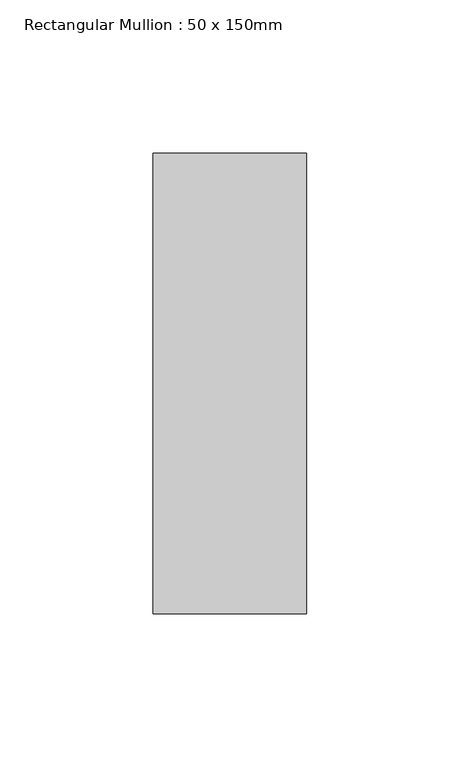
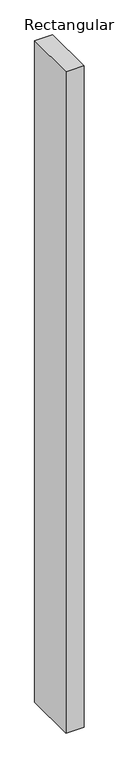
"""IFC4 building model written with IfcOpenShell, lengths in millimetres: member geometry, Rectangular Mullion : 50 x 150mm."""

from ifc_helpers import new_model, si_unit, frame, origin, place, context, project, spatial, polyline, outline, extrude, source, transform, mapped, element, save


def rectangular_mullion_50_x_150mm_a16d5dba(model_context):
    return source(origin(), model_context, "Body", "SweptSolid", [
        extrude(outline(polyline([(25.0, 75.0), (25.0, -75.0), (-25.0, -75.0), (-25.0, 75.0), (25.0, 75.0)])), frame((0.0, 0.0, -1940.4113705), z_axis=(0.0, 0.0, 1.0), x_axis=(1.0, 0.0, 0.0)), (0.0, 0.0, 1.0), 1940.4113705),
    ])


if __name__ == "__main__":
    model = new_model("IFC4")
    model_context = context("Model", 3, world=origin())
    ifc_project = project(units=[si_unit("LENGTHUNIT", "METRE", prefix="MILLI")], contexts=[model_context])
    site = spatial("IfcSite", under=ifc_project)
    building = spatial("IfcBuilding", under=site)
    placement = place(None, origin())
    rectangular_mullion_50_x_150mm_shape = rectangular_mullion_50_x_150mm_a16d5dba(model_context)
    element("IfcMember", 1, ObjectType="Rectangular Mullion : 50 x 150mm", at=placement, inside=building, context=model_context, shape_type="MappedRepresentation", body=[
        mapped(rectangular_mullion_50_x_150mm_shape, transform((0.0, 0.0, 0.0), x_axis=(1.0, 0.0, 0.0), y_axis=(0.0, 1.0, 0.0), z_axis=(0.0, 0.0, 1.0))),
    ])
    save(model, "model.ifc")

# Revit data of these elements
# Type "Rectangular Mullion : 50 x 150mm"
#   built-in parameter 1007304 = 0.492126 (stored number, unit not read)
#   built-in parameter 1007301 = 0.082021 (stored number, unit not read)
#   built-in parameter 1007300 = 0.082021 (stored number, unit not read)
# Element 1 (IfcMember, "Rectangular Mullion : 50 x 150mm")
#   Materials on its faces: "Aluminium"
# Materials
#   "Aluminium": class "Metal", colour RGB 247 247 247, transparency 0, Description = "Aluminium 6061", Cost = 0
